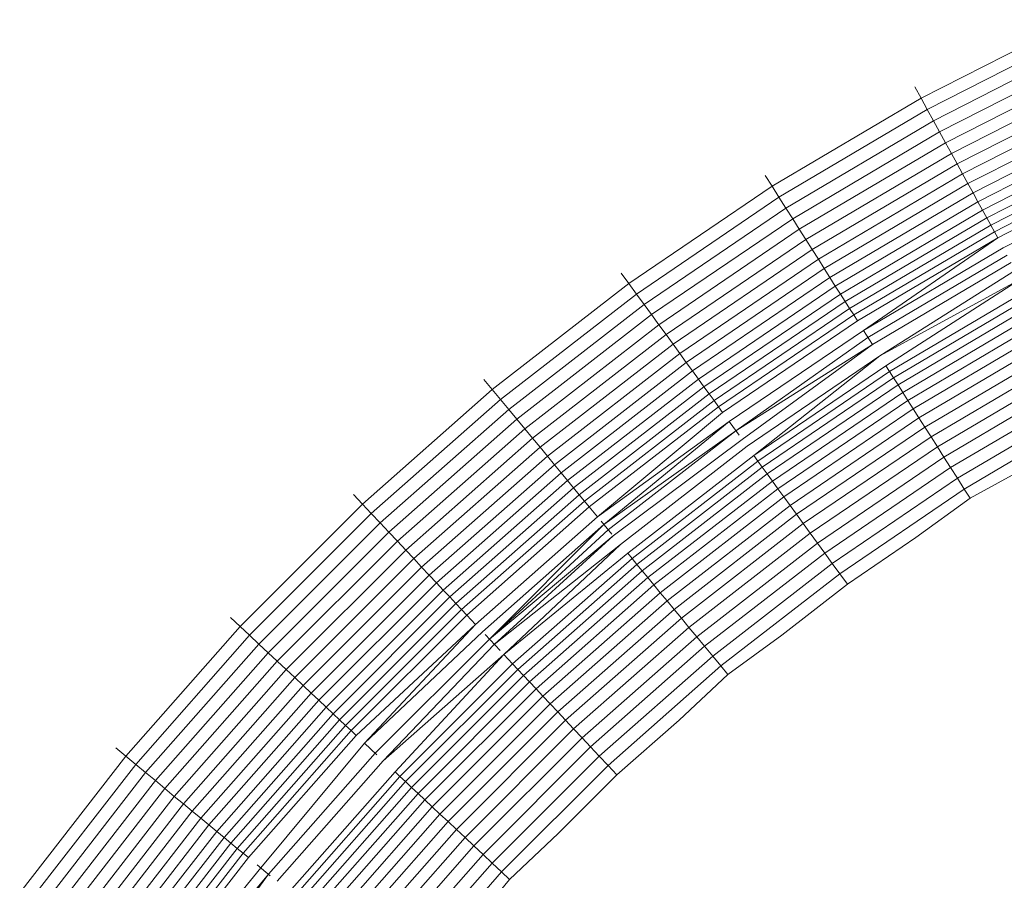
# Model space of a CAD drawing. Units: inches. Extents: x 64 to 1167, y 117 to 939.
# Tile 46 of 56: x 1129.8596 to 1130.0344, y 501.2323 to 501.3851. Entities that reach past the tile are written whole.
import ezdxf

# ---------------------------------------------------------------- set-up
doc = ezdxf.new("R2010")
doc.units = ezdxf.units.IN
doc.header["$MEASUREMENT"] = 0
doc.layers.add('A-FLOR-FIXT', color=8, linetype='Continuous', lineweight=18)

msp = doc.modelspace()

# ---------------------------------------------------------------- linework, layer by layer
at = {"layer": 'A-FLOR-FIXT'}
for p, q in [((1130.04699, 501.38507), (1130.01963, 501.37113)), ((1130.04797, 501.38299), (1130.02073, 501.36911)), ((1130.04894, 501.38093), (1130.02183, 501.36712)), ((1130.0499, 501.37889), (1130.02291, 501.36515)), ((1130.05084, 501.37689), (1130.02398, 501.36321)), ((1130.05176, 501.37494), (1130.02502, 501.36131)), ((1130.01963, 501.37113), (1130.01851, 501.37315)), ((1130.05265, 501.37304), (1130.02603, 501.35947)), ((1130.01963, 501.37113), (1129.99319, 501.35549)), ((1130.02073, 501.36911), (1130.01963, 501.37113)), ((1130.05352, 501.37119), (1130.02701, 501.35769)), ((1130.02073, 501.36911), (1129.99442, 501.35355)), ((1130.02183, 501.36712), (1130.02073, 501.36911)), ((1130.05436, 501.36942), (1130.02796, 501.35597)), ((1130.02183, 501.36712), (1129.99564, 501.35163)), ((1130.02291, 501.36515), (1130.02183, 501.36712)), ((1130.05516, 501.36772), (1130.02886, 501.35432)), ((1130.02291, 501.36515), (1129.99685, 501.34973)), ((1130.02398, 501.36321), (1130.02291, 501.36515)), ((1130.05592, 501.3661), (1130.02972, 501.35276)), ((1130.02398, 501.36321), (1129.99803, 501.34786)), ((1130.02502, 501.36131), (1130.02398, 501.36321)), ((1130.05663, 501.36458), (1130.03054, 501.35128)), ((1130.05731, 501.36315), (1130.0313, 501.3499)), ((1130.02502, 501.36131), (1129.99919, 501.34604)), ((1130.02603, 501.35947), (1130.02502, 501.36131)), ((1130.05793, 501.36182), (1130.032, 501.34861)), ((1130.02603, 501.35947), (1130.00032, 501.34426)), ((1130.02701, 501.35769), (1130.02603, 501.35947)), ((1130.0585, 501.36061), (1130.03265, 501.34744)), ((1130.05902, 501.3595), (1130.03324, 501.34637)), ((1130.02701, 501.35769), (1130.00141, 501.34254)), ((1130.02796, 501.35597), (1130.02701, 501.35769)), ((1130.05989, 501.35766), (1130.03422, 501.34458)), ((1129.99319, 501.35549), (1129.99195, 501.35744)), ((1130.02796, 501.35597), (1130.00246, 501.34089)), ((1130.02886, 501.35432), (1130.02796, 501.35597)), ((1129.99319, 501.35549), (1129.96779, 501.33823)), ((1129.99442, 501.35355), (1129.99319, 501.35549)), ((1130.02886, 501.35432), (1130.00346, 501.3393)), ((1130.02972, 501.35276), (1130.02886, 501.35432)), ((1129.99442, 501.35355), (1129.96914, 501.33637)), ((1129.99564, 501.35163), (1129.99442, 501.35355)), ((1130.02972, 501.35276), (1130.00442, 501.33779)), ((1130.03054, 501.35128), (1130.02972, 501.35276)), ((1129.99564, 501.35163), (1129.97048, 501.33453)), ((1129.99685, 501.34973), (1129.99564, 501.35163)), ((1130.03054, 501.35128), (1130.00532, 501.33637)), ((1130.0313, 501.3499), (1130.03054, 501.35128)), ((1129.99685, 501.34973), (1129.9718, 501.33271)), ((1129.99803, 501.34786), (1129.99685, 501.34973)), ((1130.0313, 501.3499), (1130.00617, 501.33504)), ((1130.032, 501.34861), (1130.0313, 501.3499)), ((1129.99803, 501.34786), (1129.9731, 501.33092)), ((1129.99919, 501.34604), (1129.99803, 501.34786)), ((1130.032, 501.34861), (1130.00696, 501.3338)), ((1130.03265, 501.34744), (1130.00768, 501.33267)), ((1130.03265, 501.34744), (1130.032, 501.34861)), ((1130.03324, 501.34637), (1130.03265, 501.34744)), ((1129.99919, 501.34604), (1129.97437, 501.32917)), ((1130.00032, 501.34426), (1129.99919, 501.34604)), ((1130.03324, 501.34637), (1130.00833, 501.33164)), ((1130.03324, 501.34637), (1130.00942, 501.32991)), ((1130.00032, 501.34426), (1129.97561, 501.32747)), ((1130.00141, 501.34254), (1130.00032, 501.34426)), ((1130.03422, 501.34458), (1130.00942, 501.32991)), ((1130.00141, 501.34254), (1129.9768, 501.32582)), ((1130.00246, 501.34089), (1130.00141, 501.34254)), ((1130.03494, 501.34328), (1130.01022, 501.32866)), ((1130.03566, 501.34196), (1130.01103, 501.32739)), ((1130.00246, 501.34089), (1129.97796, 501.32423)), ((1130.00346, 501.3393), (1130.00246, 501.34089)), ((1130.03642, 501.34058), (1130.0123, 501.32538)), ((1129.96779, 501.33823), (1129.96643, 501.3401)), ((1130.00346, 501.3393), (1129.97906, 501.32272)), ((1130.00442, 501.33779), (1130.00346, 501.3393)), ((1130.03727, 501.33903), (1130.0123, 501.32538)), ((1130.03727, 501.33903), (1130.0134, 501.32365)), ((1129.96779, 501.33823), (1129.94352, 501.31941)), ((1129.96914, 501.33637), (1129.96779, 501.33823)), ((1130.00442, 501.33779), (1129.98011, 501.32127)), ((1130.00532, 501.33637), (1130.00442, 501.33779)), ((1130.03838, 501.33701), (1130.01405, 501.32262)), ((1129.96914, 501.33637), (1129.94498, 501.31763)), ((1129.97048, 501.33453), (1129.96914, 501.33637)), ((1130.00532, 501.33637), (1129.9811, 501.31991)), ((1130.00617, 501.33504), (1129.98203, 501.31863)), ((1130.00617, 501.33504), (1130.00532, 501.33637)), ((1130.00696, 501.3338), (1130.00617, 501.33504)), ((1130.03903, 501.33583), (1130.01477, 501.32149)), ((1129.97048, 501.33453), (1129.94644, 501.31588)), ((1129.9718, 501.33271), (1129.97048, 501.33453)), ((1130.00696, 501.3338), (1129.98289, 501.31745)), ((1130.00768, 501.33267), (1130.00696, 501.3338)), ((1130.03973, 501.33455), (1130.01556, 501.32025)), ((1130.0405, 501.33316), (1130.0164, 501.31892)), ((1129.9718, 501.33271), (1129.94787, 501.31415)), ((1129.9731, 501.33092), (1129.9718, 501.33271)), ((1130.00768, 501.33267), (1129.98368, 501.31636)), ((1130.00833, 501.33164), (1129.9844, 501.31537)), ((1130.00833, 501.33164), (1130.00768, 501.33267)), ((1130.04131, 501.33169), (1130.01731, 501.31749)), ((1129.9731, 501.33092), (1129.94928, 501.31244)), ((1129.97437, 501.32917), (1129.9731, 501.33092)), ((1130.00942, 501.32991), (1129.9856, 501.31372)), ((1130.00942, 501.32991), (1130.01103, 501.32739)), ((1130.04217, 501.33012), (1130.01826, 501.31599)), ((1129.97437, 501.32917), (1129.95066, 501.31078)), ((1129.97561, 501.32747), (1129.97437, 501.32917)), ((1130.01022, 501.32866), (1129.98678, 501.31209)), ((1130.04307, 501.32848), (1130.01927, 501.3144)), ((1129.97561, 501.32747), (1129.952, 501.30916)), ((1129.9768, 501.32582), (1129.97561, 501.32747)), ((1130.01103, 501.32739), (1129.98678, 501.31209)), ((1130.01103, 501.32739), (1129.98788, 501.31057)), ((1130.04402, 501.32676), (1130.02032, 501.31274)), ((1129.9768, 501.32582), (1129.9533, 501.30759)), ((1129.97796, 501.32423), (1129.9768, 501.32582)), ((1130.0123, 501.32538), (1129.98875, 501.30937)), ((1130.0123, 501.32538), (1129.98995, 501.30772)), ((1130.045, 501.32497), (1130.02141, 501.31102)), ((1129.97796, 501.32423), (1129.95455, 501.30608)), ((1129.97906, 501.32272), (1129.95574, 501.30463)), ((1129.97906, 501.32272), (1129.97796, 501.32423)), ((1129.98011, 501.32127), (1129.97906, 501.32272)), ((1130.0134, 501.32365), (1129.98995, 501.30772)), ((1130.01405, 501.32262), (1130.0134, 501.32365)), ((1130.04601, 501.32313), (1130.02254, 501.30925)), ((1129.94352, 501.31941), (1129.94205, 501.32118)), ((1129.98011, 501.32127), (1129.95688, 501.30325)), ((1129.9811, 501.31991), (1129.98011, 501.32127)), ((1130.01405, 501.32262), (1129.99067, 501.30673)), ((1130.01477, 501.32149), (1129.99146, 501.30564)), ((1130.01477, 501.32149), (1130.01405, 501.32262)), ((1130.01556, 501.32025), (1130.01477, 501.32149)), ((1130.04705, 501.32124), (1130.0237, 501.30742)), ((1129.94352, 501.31941), (1129.92048, 501.29909)), ((1129.94498, 501.31763), (1129.94352, 501.31941)), ((1129.9811, 501.31991), (1129.95796, 501.30196)), ((1129.98203, 501.31863), (1129.9811, 501.31991)), ((1130.01556, 501.32025), (1129.99232, 501.30446)), ((1130.0164, 501.31892), (1130.01556, 501.32025)), ((1130.04812, 501.3193), (1130.02488, 501.30556)), ((1129.94498, 501.31763), (1129.92205, 501.29742)), ((1129.94644, 501.31588), (1129.94498, 501.31763)), ((1129.98203, 501.31863), (1129.95896, 501.30074)), ((1129.98289, 501.31745), (1129.9599, 501.29961)), ((1129.98289, 501.31745), (1129.98203, 501.31863)), ((1129.98368, 501.31636), (1129.98289, 501.31745)), ((1130.0164, 501.31892), (1129.99325, 501.30318)), ((1130.01731, 501.31749), (1129.99424, 501.30182)), ((1130.01731, 501.31749), (1130.0164, 501.31892)), ((1130.01826, 501.31599), (1130.01731, 501.31749)), ((1129.94644, 501.31588), (1129.92361, 501.29576)), ((1129.94787, 501.31415), (1129.94644, 501.31588)), ((1129.98368, 501.31636), (1129.96075, 501.29857)), ((1129.9844, 501.31537), (1129.98368, 501.31636)), ((1130.01826, 501.31599), (1129.99529, 501.30037)), ((1130.01927, 501.3144), (1130.01826, 501.31599)), ((1130.0492, 501.31733), (1130.02608, 501.30366)), ((1129.94787, 501.31415), (1129.92515, 501.29412)), ((1129.94928, 501.31244), (1129.94787, 501.31415)), ((1129.9844, 501.31537), (1129.96222, 501.2968)), ((1130.01927, 501.3144), (1129.99639, 501.29886)), ((1130.02032, 501.31274), (1130.01927, 501.3144)), ((1130.0503, 501.31533), (1130.02731, 501.30173)), ((1129.94928, 501.31244), (1129.92667, 501.29251)), ((1129.95066, 501.31078), (1129.94928, 501.31244)), ((1129.9856, 501.31372), (1129.96222, 501.2968)), ((1129.9856, 501.31372), (1129.96335, 501.29543)), ((1129.9856, 501.31372), (1129.98735, 501.3113)), ((1130.02032, 501.31274), (1129.99755, 501.29727)), ((1130.02141, 501.31102), (1130.02032, 501.31274)), ((1129.95066, 501.31078), (1129.92815, 501.29093)), ((1129.952, 501.30916), (1129.95066, 501.31078)), ((1129.98678, 501.31209), (1129.96335, 501.29543)), ((1129.98678, 501.31209), (1129.96411, 501.29451)), ((1129.98788, 501.31057), (1129.96498, 501.29347)), ((1130.02141, 501.31102), (1129.99874, 501.29562)), ((1130.02254, 501.30925), (1130.02141, 501.31102)), ((1129.952, 501.30916), (1129.92959, 501.2894)), ((1129.9533, 501.30759), (1129.952, 501.30916)), ((1129.98875, 501.30937), (1129.96626, 501.29192)), ((1130.02254, 501.30925), (1129.99998, 501.29392)), ((1130.0237, 501.30742), (1130.02254, 501.30925)), ((1129.9533, 501.30759), (1129.93098, 501.28791)), ((1129.95455, 501.30608), (1129.9533, 501.30759)), ((1129.98995, 501.30772), (1129.96756, 501.29035)), ((1129.99067, 501.30673), (1129.98995, 501.30772)), ((1130.0237, 501.30742), (1130.00125, 501.29217)), ((1130.02488, 501.30556), (1130.0237, 501.30742)), ((1129.95455, 501.30608), (1129.93232, 501.28648)), ((1129.95574, 501.30463), (1129.95455, 501.30608)), ((1129.99067, 501.30673), (1129.96834, 501.28941)), ((1129.99146, 501.30564), (1129.96919, 501.28837)), ((1129.99146, 501.30564), (1129.99067, 501.30673)), ((1129.99232, 501.30446), (1129.99146, 501.30564)), ((1130.02488, 501.30556), (1130.00255, 501.29038)), ((1130.02608, 501.30366), (1130.02488, 501.30556)), ((1130.03874, 501.30583), (1130.02834, 501.30011)), ((1129.95574, 501.30463), (1129.93361, 501.28512)), ((1129.95688, 501.30325), (1129.95574, 501.30463)), ((1129.99232, 501.30446), (1129.97013, 501.28724)), ((1129.99325, 501.30318), (1129.99232, 501.30446)), ((1130.02608, 501.30366), (1130.00387, 501.28856)), ((1130.02731, 501.30173), (1130.02608, 501.30366)), ((1129.95688, 501.30325), (1129.93483, 501.28381)), ((1129.95796, 501.30196), (1129.93598, 501.28259)), ((1129.95796, 501.30196), (1129.95688, 501.30325)), ((1129.95896, 501.30074), (1129.95796, 501.30196)), ((1129.99325, 501.30318), (1129.97113, 501.28603)), ((1129.99424, 501.30182), (1129.97221, 501.28473)), ((1129.99424, 501.30182), (1129.99325, 501.30318)), ((1129.99529, 501.30037), (1129.99424, 501.30182)), ((1130.02731, 501.30173), (1130.00521, 501.28672)), ((1130.02834, 501.30011), (1130.02731, 501.30173)), ((1129.9189, 501.30078), (1129.92048, 501.29909)), ((1129.95896, 501.30074), (1129.93707, 501.28143)), ((1129.9599, 501.29961), (1129.95896, 501.30074)), ((1129.99529, 501.30037), (1129.97335, 501.28335)), ((1129.99639, 501.29886), (1129.99529, 501.30037)), ((1130.02834, 501.30011), (1130.01873, 501.29313)), ((1129.92048, 501.29909), (1129.89876, 501.27738)), ((1129.92048, 501.29909), (1129.92205, 501.29742)), ((1129.9599, 501.29961), (1129.93807, 501.28037)), ((1129.96075, 501.29857), (1129.93899, 501.27939)), ((1129.96075, 501.29857), (1129.9599, 501.29961)), ((1129.96222, 501.2968), (1129.96075, 501.29857)), ((1129.99639, 501.29886), (1129.97454, 501.28191)), ((1129.99755, 501.29727), (1129.99639, 501.29886)), ((1129.92205, 501.29742), (1129.90044, 501.2758)), ((1129.92205, 501.29742), (1129.92361, 501.29576)), ((1129.96222, 501.2968), (1129.94057, 501.2777)), ((1129.99755, 501.29727), (1129.97579, 501.28039)), ((1129.99874, 501.29562), (1129.99755, 501.29727)), ((1129.92361, 501.29576), (1129.9021, 501.27424)), ((1129.92361, 501.29576), (1129.92515, 501.29412)), ((1129.96335, 501.29543), (1129.94178, 501.27642)), ((1129.96335, 501.29543), (1129.94301, 501.27511)), ((1129.96283, 501.29606), (1129.96474, 501.29376)), ((1129.99874, 501.29562), (1129.97709, 501.27882)), ((1129.99998, 501.29392), (1129.99874, 501.29562)), ((1129.92515, 501.29412), (1129.90374, 501.2727)), ((1129.92515, 501.29412), (1129.92667, 501.29251)), ((1129.96411, 501.29451), (1129.94301, 501.27511)), ((1129.96498, 501.29347), (1129.94301, 501.27511)), ((1129.96498, 501.29347), (1129.94388, 501.27417)), ((1129.99998, 501.29392), (1129.97843, 501.2772)), ((1130.00125, 501.29217), (1129.99998, 501.29392)), ((1130.01873, 501.29313), (1130.00656, 501.28486)), ((1129.92667, 501.29251), (1129.90535, 501.27119)), ((1129.92667, 501.29251), (1129.92815, 501.29093)), ((1129.96626, 501.29192), (1129.94388, 501.27417)), ((1129.96626, 501.29192), (1129.94555, 501.2724)), ((1130.00125, 501.29217), (1129.97981, 501.27554)), ((1130.00255, 501.29038), (1130.00125, 501.29217)), ((1129.92815, 501.29093), (1129.90693, 501.26971)), ((1129.92815, 501.29093), (1129.92959, 501.2894)), ((1129.96756, 501.29035), (1129.94555, 501.2724)), ((1129.96834, 501.28941), (1129.96756, 501.29035)), ((1130.00255, 501.29038), (1129.98122, 501.27384)), ((1130.00387, 501.28856), (1130.00255, 501.29038)), ((1129.92959, 501.2894), (1129.90846, 501.26827)), ((1129.93098, 501.28791), (1129.90994, 501.26688)), ((1129.92959, 501.2894), (1129.93098, 501.28791)), ((1129.93098, 501.28791), (1129.93232, 501.28648)), ((1129.96834, 501.28941), (1129.94713, 501.27071)), ((1129.96919, 501.28837), (1129.94805, 501.26973)), ((1129.96919, 501.28837), (1129.96834, 501.28941)), ((1129.97013, 501.28724), (1129.96919, 501.28837)), ((1130.00387, 501.28856), (1129.98265, 501.2721)), ((1130.00521, 501.28672), (1130.00387, 501.28856)), ((1129.93232, 501.28648), (1129.91137, 501.26554)), ((1129.93232, 501.28648), (1129.93361, 501.28512)), ((1129.97013, 501.28724), (1129.94906, 501.26867)), ((1129.97113, 501.28603), (1129.95014, 501.26752)), ((1129.97113, 501.28603), (1129.97013, 501.28724)), ((1129.97221, 501.28473), (1129.97113, 501.28603)), ((1130.00521, 501.28672), (1129.9841, 501.27035)), ((1130.00656, 501.28486), (1130.00521, 501.28672)), ((1129.93361, 501.28512), (1129.91274, 501.26425)), ((1129.93361, 501.28512), (1129.93483, 501.28381)), ((1129.97221, 501.28473), (1129.95129, 501.26629)), ((1129.97335, 501.28335), (1129.97221, 501.28473)), ((1130.00656, 501.28486), (1129.99494, 501.27584)), ((1129.93483, 501.28381), (1129.91404, 501.26303)), ((1129.93598, 501.28259), (1129.91527, 501.26187)), ((1129.93598, 501.28259), (1129.93483, 501.28381)), ((1129.93707, 501.28143), (1129.93598, 501.28259)), ((1129.97335, 501.28335), (1129.95251, 501.26499)), ((1129.97454, 501.28191), (1129.97335, 501.28335)), ((1129.93707, 501.28143), (1129.91642, 501.26079)), ((1129.93807, 501.28037), (1129.93707, 501.28143)), ((1129.97454, 501.28191), (1129.9538, 501.26362)), ((1129.97579, 501.28039), (1129.97454, 501.28191)), ((1129.93807, 501.28037), (1129.91749, 501.25979)), ((1129.93899, 501.27939), (1129.91847, 501.25887)), ((1129.93899, 501.27939), (1129.93807, 501.28037)), ((1129.94057, 501.2777), (1129.93899, 501.27939)), ((1129.97579, 501.28039), (1129.95514, 501.26219)), ((1129.97709, 501.27882), (1129.97579, 501.28039)), ((1129.89876, 501.27738), (1129.87845, 501.25434)), ((1129.89708, 501.27896), (1129.89876, 501.27738)), ((1129.89876, 501.27738), (1129.90044, 501.2758)), ((1129.94057, 501.2777), (1129.91936, 501.25803)), ((1129.94057, 501.2777), (1129.92085, 501.25664)), ((1129.97709, 501.27882), (1129.95653, 501.2607)), ((1129.97843, 501.2772), (1129.97709, 501.27882)), ((1129.90044, 501.2758), (1129.88022, 501.25287)), ((1129.90044, 501.2758), (1129.9021, 501.27424)), ((1129.94178, 501.27642), (1129.92085, 501.25664)), ((1129.94224, 501.27593), (1129.9449, 501.27309)), ((1129.97843, 501.2772), (1129.95797, 501.25917)), ((1129.97981, 501.27554), (1129.95945, 501.25759)), ((1129.97981, 501.27554), (1129.97843, 501.2772)), ((1129.98122, 501.27384), (1129.97981, 501.27554)), ((1129.99494, 501.27584), (1129.98533, 501.26886)), ((1129.9021, 501.27424), (1129.88198, 501.25142)), ((1129.9021, 501.27424), (1129.90374, 501.2727)), ((1129.94301, 501.27511), (1129.92275, 501.25485)), ((1129.94388, 501.27417), (1129.92417, 501.25352)), ((1129.98122, 501.27384), (1129.96097, 501.25598)), ((1129.98265, 501.2721), (1129.98122, 501.27384)), ((1129.90374, 501.2727), (1129.88371, 501.24999)), ((1129.90374, 501.2727), (1129.90535, 501.27119)), ((1129.94555, 501.2724), (1129.92417, 501.25352)), ((1129.94555, 501.2724), (1129.92626, 501.25156)), ((1129.94555, 501.2724), (1129.94713, 501.27071)), ((1129.98265, 501.2721), (1129.96251, 501.25434)), ((1129.9841, 501.27035), (1129.98265, 501.2721)), ((1129.90535, 501.27119), (1129.88542, 501.24858)), ((1129.90535, 501.27119), (1129.90693, 501.26971)), ((1129.94713, 501.27071), (1129.92714, 501.25073)), ((1129.94713, 501.27071), (1129.94805, 501.26973)), ((1129.9841, 501.27035), (1129.96407, 501.25268)), ((1129.98533, 501.26886), (1129.9841, 501.27035)), ((1129.90693, 501.26971), (1129.88708, 501.2472)), ((1129.90693, 501.26971), (1129.90846, 501.26827)), ((1129.94805, 501.26973), (1129.92812, 501.24981)), ((1129.94906, 501.26867), (1129.92919, 501.2488)), ((1129.94805, 501.26973), (1129.94906, 501.26867)), ((1129.94906, 501.26867), (1129.95014, 501.26752)), ((1129.98533, 501.26886), (1129.97668, 501.26074)), ((1129.90846, 501.26827), (1129.8887, 501.24586)), ((1129.90994, 501.26688), (1129.89027, 501.24456)), ((1129.90846, 501.26827), (1129.90994, 501.26688)), ((1129.90994, 501.26688), (1129.91137, 501.26554)), ((1129.95014, 501.26752), (1129.93034, 501.24772)), ((1129.95014, 501.26752), (1129.95129, 501.26629)), ((1129.91137, 501.26554), (1129.89178, 501.24331)), ((1129.91137, 501.26554), (1129.91274, 501.26425)), ((1129.95129, 501.26629), (1129.93157, 501.24657)), ((1129.95251, 501.26499), (1129.93287, 501.24535)), ((1129.95129, 501.26629), (1129.95251, 501.26499)), ((1129.95251, 501.26499), (1129.9538, 501.26362)), ((1129.91274, 501.26425), (1129.89323, 501.24212)), ((1129.91274, 501.26425), (1129.91404, 501.26303)), ((1129.9538, 501.26362), (1129.93424, 501.24406)), ((1129.9538, 501.26362), (1129.95514, 501.26219)), ((1129.91404, 501.26303), (1129.8946, 501.24098)), ((1129.91527, 501.26187), (1129.8959, 501.2399)), ((1129.91404, 501.26303), (1129.91527, 501.26187)), ((1129.91527, 501.26187), (1129.91642, 501.26079)), ((1129.95514, 501.26219), (1129.93567, 501.24272)), ((1129.95514, 501.26219), (1129.95653, 501.2607)), ((1129.91642, 501.26079), (1129.89712, 501.2389)), ((1129.91749, 501.25979), (1129.89825, 501.23796)), ((1129.91642, 501.26079), (1129.91749, 501.25979)), ((1129.91749, 501.25979), (1129.91847, 501.25887)), ((1129.95653, 501.2607), (1129.93716, 501.24132)), ((1129.95653, 501.2607), (1129.95797, 501.25917)), ((1129.97668, 501.26074), (1129.96564, 501.25101)), ((1129.91847, 501.25887), (1129.89928, 501.23711)), ((1129.91936, 501.25803), (1129.90022, 501.23633)), ((1129.91847, 501.25887), (1129.91936, 501.25803)), ((1129.95797, 501.25917), (1129.93869, 501.23988)), ((1129.95797, 501.25917), (1129.95945, 501.25759)), ((1129.92085, 501.25664), (1129.90242, 501.23451)), ((1129.92085, 501.25664), (1129.92303, 501.25459)), ((1129.95945, 501.25759), (1129.94027, 501.2384)), ((1129.95945, 501.25759), (1129.96097, 501.25598)), ((1129.87845, 501.25434), (1129.87667, 501.25581)), ((1129.92275, 501.25485), (1129.90381, 501.23336)), ((1129.96097, 501.25598), (1129.94188, 501.23689)), ((1129.96097, 501.25598), (1129.96251, 501.25434)), ((1129.87845, 501.25434), (1129.85963, 501.23007)), ((1129.88022, 501.25287), (1129.86149, 501.22872)), ((1129.88022, 501.25287), (1129.87845, 501.25434)), ((1129.88198, 501.25142), (1129.88022, 501.25287)), ((1129.92417, 501.25352), (1129.90531, 501.23212)), ((1129.96251, 501.25434), (1129.94352, 501.23535)), ((1129.96251, 501.25434), (1129.96407, 501.25268)), ((1129.88198, 501.25142), (1129.86333, 501.22738)), ((1129.88371, 501.24999), (1129.88198, 501.25142)), ((1129.92626, 501.25156), (1129.90751, 501.2303)), ((1129.92714, 501.25073), (1129.92626, 501.25156)), ((1129.96407, 501.25268), (1129.94518, 501.23379)), ((1129.96564, 501.25101), (1129.95523, 501.2406)), ((1129.96407, 501.25268), (1129.96564, 501.25101)), ((1129.88371, 501.24999), (1129.86515, 501.22606)), ((1129.88542, 501.24858), (1129.88371, 501.24999)), ((1129.92714, 501.25073), (1129.90845, 501.22952)), ((1129.92812, 501.24981), (1129.90949, 501.22867)), ((1129.92812, 501.24981), (1129.92714, 501.25073)), ((1129.92919, 501.2488), (1129.92812, 501.24981)), ((1129.88542, 501.24858), (1129.86694, 501.22476)), ((1129.88708, 501.2472), (1129.88542, 501.24858)), ((1129.92919, 501.2488), (1129.91062, 501.22773)), ((1129.93034, 501.24772), (1129.91183, 501.22673)), ((1129.93034, 501.24772), (1129.92919, 501.2488)), ((1129.93157, 501.24657), (1129.93034, 501.24772)), ((1129.88708, 501.2472), (1129.86869, 501.22349)), ((1129.8887, 501.24586), (1129.87039, 501.22225)), ((1129.8887, 501.24586), (1129.88708, 501.2472)), ((1129.89027, 501.24456), (1129.8887, 501.24586)), ((1129.93157, 501.24657), (1129.91313, 501.22565)), ((1129.93287, 501.24535), (1129.93157, 501.24657)), ((1129.89027, 501.24456), (1129.87204, 501.22106)), ((1129.89178, 501.24331), (1129.89027, 501.24456)), ((1129.93287, 501.24535), (1129.91451, 501.22451)), ((1129.93424, 501.24406), (1129.91595, 501.22332)), ((1129.93424, 501.24406), (1129.93287, 501.24535)), ((1129.93567, 501.24272), (1129.93424, 501.24406)), ((1129.89178, 501.24331), (1129.87362, 501.2199)), ((1129.89323, 501.24212), (1129.89178, 501.24331)), ((1129.93567, 501.24272), (1129.91746, 501.22207)), ((1129.93716, 501.24132), (1129.93567, 501.24272)), ((1129.89323, 501.24212), (1129.87514, 501.2188)), ((1129.8946, 501.24098), (1129.87659, 501.21775)), ((1129.8946, 501.24098), (1129.89323, 501.24212)), ((1129.8959, 501.2399), (1129.8946, 501.24098)), ((1129.93716, 501.24132), (1129.91903, 501.22077)), ((1129.93869, 501.23988), (1129.93716, 501.24132)), ((1129.95523, 501.2406), (1129.94658, 501.23247)), ((1129.8959, 501.2399), (1129.87795, 501.21676)), ((1129.89712, 501.2389), (1129.87923, 501.21583)), ((1129.89712, 501.2389), (1129.8959, 501.2399)), ((1129.89825, 501.23796), (1129.89712, 501.2389)), ((1129.93869, 501.23988), (1129.92065, 501.21943)), ((1129.94027, 501.2384), (1129.93869, 501.23988)), ((1129.89825, 501.23796), (1129.88041, 501.21497)), ((1129.89928, 501.23711), (1129.8815, 501.21418)), ((1129.89928, 501.23711), (1129.89825, 501.23796)), ((1129.90022, 501.23633), (1129.89928, 501.23711)), ((1129.94027, 501.2384), (1129.92232, 501.21805)), ((1129.94188, 501.23689), (1129.94027, 501.2384)), ((1129.90022, 501.23633), (1129.88249, 501.21346)), ((1129.94188, 501.23689), (1129.92402, 501.21664)), ((1129.94352, 501.23535), (1129.92576, 501.21521)), ((1129.94352, 501.23535), (1129.94188, 501.23689)), ((1129.94518, 501.23379), (1129.94352, 501.23535)), ((1129.90242, 501.23451), (1129.88414, 501.21226)), ((1129.9018, 501.23503), (1129.9041, 501.23312)), ((1129.94518, 501.23379), (1129.92751, 501.21375)), ((1129.94658, 501.23247), (1129.94518, 501.23379)), ((1129.90381, 501.23336), (1129.88534, 501.21139)), ((1129.90381, 501.23336), (1129.88686, 501.21029)), ((1129.94658, 501.23247), (1129.93901, 501.22333))]:
    msp.add_line(p, q, dxfattribs=at)

doc.saveas('drawing.dxf')
